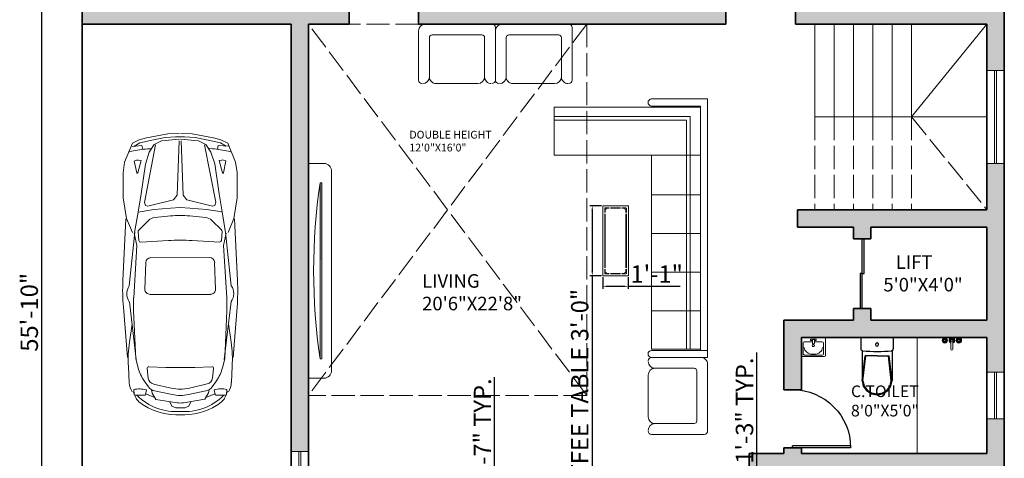
# Model space of a CAD drawing. Units: inches. Extents: x 4606 to 5879, y 1332 to 2209.
# Tile 3 of 7: x 4626 to 5136, y 1671 to 1897. Entities that reach past the tile are written whole.
import ezdxf

# ---------------------------------------------------------------- set-up
doc = ezdxf.new("R2010")
doc.units = ezdxf.units.IN
doc.linetypes.add('ACAD_ISO02W100', pattern=[15, 12, -3])
for name, color, linetype, lineweight in [('A-ANNO-DIMS', 2, 'Continuous', 18), ('A-AREA-IDEN', 7, 'Continuous', 18), ('A-DOOR', 4, 'Continuous', 25), ('A-EQPM', 9, 'Continuous', 18), ('A-FLOR-OVHD', 8, 'ACAD_ISO02W100', 13), ('A-FLOR-STRS', 7, 'Continuous', 20), ('A-FLOR-STRS-OVHD', 8, 'ACAD_ISO02W100', 13), ('A-FURN', 8, 'Continuous', 18), ('A-SITE-PARK', 8, 'Continuous', 13), ('A-WALL', 7, 'Continuous', 35), ('A-WALL-PATT', 252, 'Continuous', 13), ('window', 130, 'Continuous', 18), ('Сантехника', 9, 'Continuous', 18)]:
    doc.layers.add(name, color=color, linetype=linetype, lineweight=lineweight)
doc.layers.add('SANTEH', color=7, linetype='Continuous')
doc.styles.get("Standard").update_dxf_attribs({"font": 'arial.ttf'})
doc.dimstyles.new('ISO-25', dxfattribs={"dimtxt": 9, "dimasz": 2.5, "dimexe": 1.25, "dimexo": 0.625, "dimtad": 1, "dimlunit": 3, "dimtxsty": 'Standard', "dimcen": 2.5, "dimadec": 0, "dimazin": 0, "dimtfac": 1, "dimtmove": 0, "dimatfit": 3, "dimfxl": 1, "dimarcsym": 0})

# ---------------------------------------------------------------- blocks, each defined once
blk = doc.blocks.new('D2')
for p, q in [((0, 30), (0, 0)), ((1, 30), (1, 0)), ((0, 0), (1, 0))]:
    blk.add_line(p, q)
blk.add_arc((0, 0), 30, 0, 90)
blk = doc.blocks.new('WC 2 Symb_109')
at = {"layer": 'SANTEH'}
for p, q in [((0, 0), (0, 380)), ((0, 380), (132, 380)), ((154, 365), (507, 365)), ((506, 365), (216, 331)), ((506, 356), (216, 322)), ((216, 190), (216, 331)), ((216, 190), (216, 49)), ((154, 15), (507, 15)), ((506, 24), (216, 58)), ((506, 15), (216, 49)), ((0, 0), (132, 0))]:
    blk.add_line(p, q, dxfattribs=at)
for points in [[(155, 360), (154, 364), (152, 368), (150, 371), (147, 374), (144, 377), (140, 379), (137, 380), (132, 380)], [(155, 20), (159, 62), (161, 105), (163, 147), (164, 190), (163, 233), (161, 275), (159, 318), (155, 360)], [(506, 24), (565, 37), (616, 73), (649, 126), (661, 190), (649, 254), (616, 307), (565, 343), (506, 356)], [(507, 15), (569, 28), (622, 66), (658, 123), (670, 190), (658, 257), (622, 314), (569, 352), (507, 365)], [(132, 0), (136, 0), (140, 1), (144, 3), (147, 6), (150, 9), (152, 12), (154, 16), (155, 20)]]:
    blk.add_lwpolyline(points, dxfattribs=at)
blk.add_lwpolyline([(84, 208), (70, 203), (65, 190), (70, 177), (84, 172), (97, 177), (102, 190), (97, 203)], close=True, dxfattribs=at)
blk = doc.blocks.new('Faucet - Bathroom top')
for p, q in [((-4.107, 0.125), (-4.375, 0.125)), ((-3.75, 0.4788), (-3.75, 0.75)), ((-3.5, 0.482), (-3.5, 0.75)), ((-3.1461, 0.125), (-2.875, 0.125)), ((3.143, 0.125), (2.875, 0.125)), ((3.5, 0.4788), (3.5, 0.75)), ((3.75, 0.482), (3.75, 0.75)), ((4.1039, 0.125), (4.375, 0.125)), ((-4.1039, -0.125), (-4.375, -0.125)), ((-3.75, -0.4821), (-3.75, -0.75)), ((-3.5, -0.4789), (-3.5, -0.75)), ((-3.143, -0.125), (-2.875, -0.125)), ((-0.5, -0.8639), (-0.5, -4.5)), ((0.5, -4.5), (0.5, -0.8631)), ((3.1461, -0.125), (2.875, -0.125)), ((3.5, -0.4821), (3.5, -0.75)), ((3.75, -0.4789), (3.75, -0.75)), ((4.107, -0.125), (4.375, -0.125))]:
    blk.add_line(p, q)
for centre, radius in [((-3.625, 0), 1.375), ((-4.625, 0), 0.2795), ((-3.625, 0), 0.5), ((-3.625, 1), 0.2795), ((-2.625, 0), 0.2795), ((0, 0), 0.5), ((3.625, 0), 1.375), ((2.625, 0), 0.2795), ((3.625, 0), 0.5), ((3.625, 1), 0.2795), ((4.625, 0), 0.2795), ((-3.625, -1), 0.2795), ((3.625, -1), 0.2795)]:
    blk.add_circle(centre, radius)
for centre, radius, start, end in [((-3.625, 0), 1, 105.2407, 164.2093), ((-3.625, 0), 1, 16.44125, 74.07887), ((0, 0), 1.5, 289.6514, 250.3603), ((0, 0), 1, 300.3431, 239.7554), ((3.625, 0), 1, 106.12, 164.0884), ((3.625, 0), 1, 16.23422, 73.90469), ((-3.625, 0), 1, 196.2342, 253.9047), ((-3.625, 0), 1, 286.12, 344.0884), ((0, -4.5), 0.5, 180, 0), ((3.625, 0), 1, 196.4413, 254.0789), ((3.625, 0), 1, 285.2407, 344.2093)]:
    blk.add_arc(centre, radius, start, end)
blk = doc.blocks.new('Rac7')
at = {"color": 0}
for p, q in [((-39501, -24232), (-39501, -23830)), ((-39474, -23808), (-38988, -23808)), ((-39457, -23859), (-39457, -24115)), ((-39032, -23838), (-39430, -23838)), ((-39221, -23855), (-39241, -23855)), ((-39005, -24115), (-39005, -23859)), ((-39005, -23859), (-39005, -23859)), ((-38961, -23830), (-38961, -24232)), ((-38961, -24232), (-39501, -24232)), ((-39430, -24136), (-39253, -24136)), ((-39297, -24164), (-39253, -24164)), ((-39297, -24194), (-39297, -24164)), ((-39165, -24194), (-39297, -24194)), ((-39253, -24186), (-39253, -24094)), ((-39253, -24186), (-39209, -24186)), ((-39209, -24186), (-39209, -24094)), ((-39209, -24136), (-39032, -24136)), ((-39209, -24164), (-39165, -24164)), ((-39165, -24164), (-39165, -24194))]:
    blk.add_line(p, q, dxfattribs=at)
at = {"color": 0, "extrusion": (0, 0, -1)}
for centre, major_axis, start_param, end_param in [((-39474, -23830), (-27, 0), 0, 1.570796), ((-39430, -23859), (-27, 0), 0, 1.570796), ((-39241, -24007), (-194, 0), 0, 1.570796), ((-39221, -24007), (-194, 0), 1.570796, 3.141593), ((-39032, -23859), (-27, 0), 1.570796, 3.141593), ((-38988, -23830), (-27, 0), 1.570796, 3.141593), ((-39430, -24115), (-27, 0), -1.570796, 0), ((-39231, -24104), (-25.3, 0), 0.552816, 2.588777), ((-39032, -24115), (-27, 0), -3.141593, -1.570796)]:
    blk.add_ellipse(centre, major_axis=major_axis, ratio=0.785714, start_param=start_param, end_param=end_param, dxfattribs=at)
blk.add_ellipse((-39231, -24048), major_axis=(-27.9, 0), ratio=0.785714, dxfattribs=at)
blk = doc.blocks.new('TABLE-30A')
at = {"color": 0, "linetype": 'ByBlock'}
for p, q in [((0, 0), (0, 0.55)), ((0, 0.55), (1.5, 0.55)), ((0.051, 0.508), (0.042, 0.499)), ((0.042, 0.499), (0.042, 0.478)), ((0.042, 0.478), (0.072, 0.478)), ((0.042, 0.478), (0.042, 0.41)), ((0.072, 0.508), (0.051, 0.508)), ((0.051, 0.478), (0.051, 0.41)), ((0.072, 0.478), (0.072, 0.508)), ((0.072, 0.508), (0.14, 0.508)), ((0.072, 0.499), (0.14, 0.499)), ((1.331, 0.508), (0.169, 0.508)), ((1.331, 0.499), (0.169, 0.499)), ((1.428, 0.508), (1.36, 0.508)), ((1.428, 0.499), (1.36, 0.499)), ((1.428, 0.508), (1.428, 0.478)), ((1.449, 0.508), (1.428, 0.508)), ((1.428, 0.478), (1.458, 0.478)), ((1.458, 0.499), (1.449, 0.508)), ((1.449, 0.478), (1.449, 0.41)), ((1.458, 0.478), (1.458, 0.499)), ((1.458, 0.478), (1.458, 0.41)), ((1.5, 0.55), (1.5, 0)), ((0.042, 0.169), (0.042, 0.381)), ((0.051, 0.169), (0.051, 0.381)), ((1.449, 0.381), (1.449, 0.169)), ((1.458, 0.381), (1.458, 0.169)), ((1.5, 0), (0, 0)), ((0.042, 0.072), (0.042, 0.14)), ((0.042, 0.072), (0.042, 0.051)), ((0.072, 0.072), (0.042, 0.072)), ((0.042, 0.051), (0.051, 0.042)), ((0.051, 0.072), (0.051, 0.14)), ((0.051, 0.042), (0.072, 0.042)), ((0.072, 0.042), (0.072, 0.072)), ((0.072, 0.051), (0.14, 0.051)), ((0.072, 0.042), (0.14, 0.042)), ((0.169, 0.051), (1.331, 0.051)), ((0.169, 0.042), (1.331, 0.042)), ((1.428, 0.051), (1.36, 0.051)), ((1.428, 0.042), (1.36, 0.042)), ((1.428, 0.072), (1.428, 0.042)), ((1.458, 0.072), (1.428, 0.072)), ((1.428, 0.042), (1.449, 0.042)), ((1.449, 0.072), (1.449, 0.14)), ((1.449, 0.042), (1.458, 0.051)), ((1.458, 0.072), (1.458, 0.14)), ((1.458, 0.051), (1.458, 0.072))]:
    blk.add_line(p, q, dxfattribs=at)
blk = doc.blocks.new('sofa-27')
at = {"color": 0, "linetype": 'ByBlock'}
for p, q in [((0.0945, 0.5198), (0.459, 0.5198)), ((-0.0591, 0.0591), (-0.0591, 0.4902)), ((0.0354, 0.1181), (0.0354, 0.4607)), ((0.518, 0.1181), (0.518, 0.4607)), ((0.6125, 0.0295), (0.6125, 0.4902)), ((0.4944, 0.0945), (0.0591, 0.0945)), ((0.583, 0), (0, 0))]:
    blk.add_line(p, q, dxfattribs=at)
for centre, radius, start, end in [((-0.0295, 0.4902), 0.0295, 90, 180), ((-0.0236, 0.4607), 0.0591, 360, 90), ((0.0945, 0.4607), 0.0591, 90, 180), ((0.459, 0.4607), 0.0591, 0, 90), ((0.5771, 0.4607), 0.0591, 90, 180), ((0.583, 0.4902), 0.0295, 0, 90), ((0.0591, 0.1181), 0.0236, 180, 270), ((0.4944, 0.1181), 0.0236, 270, 0), ((0, 0.0591), 0.0591, 180, 270), ((0.583, 0.0295), 0.0295, 270, 0)]:
    blk.add_arc(centre, radius, start, end, dxfattribs=at)
blk = doc.blocks.new('A$C4A3239E3')
for p, q in [((1.251, 1.634), (2.152, 1.68)), ((2.545, 1.674), (3.282, 1.615)), ((3.41, 1.602), (3.649, 1.59)), ((0.136, 1.429), (0.187, 1.515)), ((0.175, 1.399), (0.187, 1.541)), ((0.266, 1.579), (0.259, 1.549)), ((0.396, 1.412), (0.388, 1.449)), ((0.39, 1.477), (0.402, 1.511)), ((0.576, 1.46), (0.396, 1.412)), ((0.402, 1.511), (0.575, 1.474)), ((1.45, 1.506), (1.149, 1.455)), ((1.272, 1.303), (1.413, 1.446)), ((1.433, 1.454), (1.567, 1.444)), ((1.443, 1.502), (2.231, 1.588)), ((1.461, 1.515), (1.641, 1.474)), ((1.641, 1.474), (2.408, 1.522)), ((2.463, 1.587), (3.312, 1.486)), ((2.597, 1.524), (3.301, 1.494)), ((2.788, 1.546), (3.057, 1.586)), ((3.301, 1.494), (3.432, 1.46)), ((3.822, 1.52), (3.752, 1.525)), ((3.781, 1.532), (3.813, 1.518)), ((3.833, 1.363), (3.833, 1.508)), ((3.838, 1.508), (3.867, 1.496)), ((0.09, 1.227), (0.136, 1.429)), ((0.231, 1.387), (0.175, 1.399)), ((0.224, 1.314), (0.221, 1.265)), ((1.59, 1.418), (1.567, 1.013)), ((1.89, 1.345), (2.279, 1.358)), ((3.416, 1.302), (3.429, 1.052)), ((3.443, 1.328), (3.584, 1.312)), ((3.622, 1.372), (3.711, 1.31)), ((3.756, 1.339), (3.823, 1.351)), ((3.814, 1.35), (3.869, 1.214)), ((0.056, 1.059), (0.09, 1.227)), ((1.207, 0.98), (1.229, 1.212)), ((1.819, 0.408), (1.818, 1.271)), ((2.356, 1.283), (2.357, 0.397)), ((3.669, 1.236), (3.73, 0.976)), ((3.753, 1.264), (3.801, 1.255)), ((3.771, 1.218), (3.825, 0.963)), ((3.801, 1.255), (3.894, 1.199)), ((3.894, 1.199), (3.945, 0.89)), ((0.048, 0.904), (0.056, 1.059)), ((3.429, 1.052), (3.429, 0.843)), ((3.929, 0.994), (3.993, 0.967)), ((3.993, 0.967), (4.017, 0.906)), ((4.017, 0.906), (4.021, 0.842)), ((0.048, 0.772), (0.057, 0.617)), ((3.43, 0.631), (3.429, 0.84)), ((3.895, 0.484), (3.945, 0.793)), ((3.994, 0.717), (4.017, 0.778)), ((4.017, 0.778), (4.021, 0.842)), ((0.057, 0.617), (0.091, 0.45)), ((1.208, 0.698), (1.23, 0.466)), ((1.591, 0.261), (1.567, 0.666)), ((3.417, 0.38), (3.43, 0.631)), ((3.67, 0.447), (3.73, 0.707)), ((3.772, 0.465), (3.825, 0.721)), ((3.929, 0.689), (3.994, 0.717)), ((0.091, 0.45), (0.137, 0.247)), ((3.802, 0.428), (3.895, 0.484)), ((3.815, 0.333), (3.869, 0.469)), ((0.232, 0.29), (0.176, 0.277)), ((0.225, 0.362), (0.222, 0.411)), ((1.273, 0.375), (1.415, 0.232)), ((1.891, 0.334), (2.28, 0.323)), ((3.444, 0.354), (3.585, 0.371)), ((3.623, 0.311), (3.712, 0.373)), ((3.754, 0.419), (3.802, 0.428)), ((3.757, 0.344), (3.824, 0.333)), ((3.834, 0.32), (3.835, 0.175)), ((0.137, 0.247), (0.188, 0.161)), ((0.176, 0.277), (0.188, 0.136)), ((0.397, 0.265), (0.389, 0.228)), ((0.391, 0.2), (0.403, 0.166)), ((0.577, 0.217), (0.397, 0.265)), ((0.403, 0.166), (0.577, 0.203)), ((1.451, 0.172), (1.15, 0.223)), ((1.434, 0.225), (1.568, 0.235)), ((1.444, 0.176), (2.233, 0.092)), ((1.462, 0.164), (1.642, 0.205)), ((1.642, 0.205), (2.409, 0.158)), ((2.464, 0.094), (3.313, 0.196)), ((2.598, 0.156), (3.302, 0.188)), ((3.302, 0.188), (3.433, 0.223)), ((3.823, 0.163), (3.753, 0.158)), ((3.783, 0.151), (3.814, 0.165)), ((3.839, 0.175), (3.868, 0.188)), ((0.268, 0.097), (0.261, 0.127)), ((1.252, 0.045), (2.154, 0)), ((2.546, 0.006), (3.283, 0.067)), ((2.789, 0.135), (3.058, 0.096)), ((3.412, 0.08), (3.651, 0.093))]:
    blk.add_line(p, q)
for points in [[(0, 0.848), (0.005, 1.016), (0.062, 1.33), (0.09, 1.438), (0.141, 1.536), (0.419, 1.653), (0.572, 1.674), (0.94, 1.674), (1.246, 1.627), (1.45, 1.541)], [(0.081, 0.844), (0.109, 1.11), (0.161, 1.218), (0.274, 1.291), (0.446, 1.347), (0.881, 1.409), (1.149, 1.455), (1.112, 1.224), (1.093, 0.981), (1.085, 0.839)], [(0.164, 1.198), (1.007, 1.364), (1.054, 1.346), (1.062, 1.312), (0.971, 0.937), (0.904, 0.882), (0.106, 0.853)], [(0, 0.828), (0.006, 0.66), (0.063, 0.346), (0.092, 0.239), (0.143, 0.14), (0.42, 0.024), (0.574, 0.003), (0.942, 0.003), (1.247, 0.051), (1.451, 0.138)], [(0.081, 0.832), (0.109, 0.566), (0.162, 0.458), (0.275, 0.386), (0.447, 0.33), (0.882, 0.268), (1.15, 0.223), (1.113, 0.454), (1.094, 0.696), (1.085, 0.839)], [(0.165, 0.478), (1.008, 0.314), (1.055, 0.332), (1.063, 0.366), (0.971, 0.741), (0.904, 0.796), (0.106, 0.823)]]:
    blk.add_lwpolyline(points)
for centre, radius, start, end in [((2.305, -1.296), 2.98, 85.3952, 92.9452), ((2.346, 1.423), 0.202, 54.6492, 124.7769), ((3.317, -0.183), 1.788, 86.9998, 98.3676), ((3.635, 1.312), 0.278, 57.3299, 87.1824), ((1.71, 1.212), 1.49, 166.9166, 176.0811), ((0.436, 1.46), 0.0497, 159.9787, 192.5384), ((0.574, 1.467), 0.00745, 284.96, 78.1125), ((1.431, 1.429), 0.0248, 85.7151, 135.3046), ((2.521, -0.262), 1.788, 87.5491, 93.6237), ((3.28, 0.883), 0.596, 55.07, 75.2551), ((4.097, 1.439), 0.356, 166.0961, 196.3535), ((3.821, 1.508), 0.0124, 0, 86.3304), ((3.247, 0.896), 0.828, 356.2451, 44.5195), ((3.809, 1.358), 0.149, 46.3836, 67.2014), ((3.618, 1.158), 0.426, 30.4577, 46.3836), ((1.378, 1.198), 0.149, 135.3046, 174.6214), ((1.565, 1.419), 0.0248, 356.7256, 85.7151), ((1.892, 1.271), 0.0745, 91.8201, 179.9989), ((2.281, 1.283), 0.0745, 359.9245, 91.8201), ((3.441, 1.304), 0.0248, 83.376, 183.115), ((3.573, 1.213), 0.0993, 13.1226, 83.376), ((3.625, 1.188), 0.149, 11.7694, 55.07), ((3.821, 1.363), 0.0124, 279.6077, 0), ((3.132, 0.872), 0.989, 358.0694, 30.4577), ((4.542, 0.842), 2.98, 176.7256, 183.3874), ((1.238, 0.839), 1.192, 176.8942, 183.2188), ((2.691, 0.84), 1.49, 174.6214, 185.4916), ((3.149, 0.841), 0.596, 346.9903, 13.1226), ((3.241, 0.841), 0.596, 348.3436, 11.7694), ((3.651, 0.841), 0.298, 350.7246, 9.3883), ((3.247, 0.786), 0.828, 315.5935, 3.8679), ((3.133, 0.809), 0.989, 329.6553, 2.0435), ((1.378, 0.48), 0.149, 185.4916, 224.8083), ((3.573, 0.469), 0.0993, 276.737, 346.9903), ((3.626, 0.495), 0.149, 305.0429, 348.3436), ((1.711, 0.467), 1.49, 184.0319, 193.1964), ((1.893, 0.409), 0.0745, 180.1141, 268.2929), ((2.282, 0.397), 0.0745, 268.2929, 0.1885), ((3.441, 0.379), 0.0248, 176.9979, 276.737), ((3.281, 0.799), 0.596, 284.8579, 305.0429), ((4.098, 0.244), 0.356, 163.7595, 194.0169), ((3.822, 0.32), 0.0124, 0.113, 80.5053), ((3.619, 0.525), 0.426, 313.7293, 329.6553), ((0.438, 0.217), 0.0497, 167.5746, 200.1342), ((0.575, 0.21), 0.00745, 282.0005, 75.153), ((1.432, 0.249), 0.0248, 224.8083, 274.3979), ((1.566, 0.26), 0.0248, 274.3979, 3.3874), ((2.518, 1.942), 1.788, 266.4893, 272.5638), ((3.822, 0.175), 0.0124, 273.7825, 0.113), ((3.81, 0.325), 0.149, 292.9116, 313.7293), ((2.301, 2.976), 2.98, 267.1678, 274.7177), ((2.347, 0.258), 0.202, 235.336, 305.4638), ((3.315, 1.865), 1.788, 261.7454, 273.1132), ((3.636, 0.371), 0.278, 272.9306, 302.783)]:
    blk.add_arc(centre, radius, start, end)
blk = doc.blocks.new('*D24')
at = {"layer": 'A-ANNO-DIMS', "color": 0, "lineweight": -2, "transparency": 16777216}
for p, q in [((4658.23, 2081.24), (4636.6, 2081.24)), ((4637.85, 2078.74), (4637.85, 1413.74)), ((4658.23, 1411.24), (4636.6, 1411.24))]:
    blk.add_line(p, q, dxfattribs=at)
at = {"layer": 'A-ANNO-DIMS', "color": 0, "transparency": 16777216}
for points in [[(4637.43, 2078.74), (4638.26, 2078.74), (4637.85, 2081.24)], [(4637.43, 1413.74), (4638.26, 1413.74), (4637.85, 1411.24)]]:
    blk.add_solid(points, dxfattribs=at)
at = {"layer": 'Defpoints', "color": 0, "transparency": 16777216}
for p in [(4658.85, 2081.24), (4637.85, 1411.24), (4658.85, 1411.24)]:
    blk.add_point(p, dxfattribs=at)
at = {"layer": 'A-ANNO-DIMS', "color": 0, "transparency": 16777216, "insert": (4632.62, 1746.24), "char_height": 9, "attachment_point": 5, "rotation": 90}
blk.add_mtext('55\'-10"', dxfattribs=at)
blk = doc.blocks.new('GLAZING-72IN')
for p, q in [((0, 0), (0, 72)), ((1, 0), (1, 72))]:
    blk.add_line(p, q)
blk = doc.blocks.new('GLAZING-24IN')
for p, q in [((0, 0), (0, 24)), ((1, 0), (1, 24))]:
    blk.add_line(p, q)
blk = doc.blocks.new('GLAZING-48IN')
for p, q in [((0, 0), (0, 48)), ((1, 0), (1, 48))]:
    blk.add_line(p, q)
blk = doc.blocks.new('LIFT-DOOR-36IN')
for p, q in [((1, 0), (1, 36)), ((2, 18), (2, 36)), ((1, 18), (0, 18)), ((0, 18), (0, 0)), ((1, 18), (2, 18))]:
    blk.add_line(p, q)
blk = doc.blocks.new('*D83')
at = {"layer": 'A-ANNO-DIMS', "color": 0, "lineweight": -2, "transparency": 16777216}
for p, q in [((5007.89, 1624.4), (5007.89, 1725.52)), ((5009.49, 1624.4), (5006.64, 1624.4)), ((5007.89, 1612.06), (5007.89, 1621.9)), ((5009.49, 1609.56), (5006.64, 1609.56))]:
    blk.add_line(p, q, dxfattribs=at)
at = {"layer": 'A-ANNO-DIMS', "color": 0, "transparency": 16777216}
for points in [[(5007.47, 1621.9), (5008.31, 1621.9), (5007.89, 1624.4)], [(5007.47, 1612.06), (5008.31, 1612.06), (5007.89, 1609.56)]]:
    blk.add_solid(points, dxfattribs=at)
at = {"layer": 'Defpoints', "color": 0, "transparency": 16777216}
for p in [(5007.89, 1624.4), (5010.11, 1624.4), (5010.11, 1609.56)]:
    blk.add_point(p, dxfattribs=at)
at = {"layer": 'A-ANNO-DIMS', "color": 0, "transparency": 16777216, "insert": (5002.61, 1676.21), "char_height": 9, "attachment_point": 5, "rotation": 90}
blk.add_mtext('CHAIR 1\'-3" TYP.', dxfattribs=at)
blk = doc.blocks.new('*D88')
at = {"layer": 'A-ANNO-DIMS', "color": 0, "lineweight": -2, "transparency": 16777216}
for p, q in [((4872.19, 1654), (4872.19, 1712.76)), ((4866.85, 1654), (4873.44, 1654)), ((4872.19, 1625.74), (4872.19, 1651.5)), ((4866.85, 1623.24), (4873.44, 1623.24))]:
    blk.add_line(p, q, dxfattribs=at)
at = {"layer": 'A-ANNO-DIMS', "color": 0, "transparency": 16777216}
for points in [[(4871.77, 1651.5), (4872.6, 1651.5), (4872.19, 1654)], [(4871.77, 1625.74), (4872.6, 1625.74), (4872.19, 1623.24)]]:
    blk.add_solid(points, dxfattribs=at)
at = {"layer": 'Defpoints', "color": 0, "transparency": 16777216}
for p in [(4866.23, 1654), (4872.19, 1654), (4866.23, 1623.24)]:
    blk.add_point(p, dxfattribs=at)
at = {"layer": 'A-ANNO-DIMS', "color": 0, "transparency": 16777216, "insert": (4867.04, 1684.63), "char_height": 9, "attachment_point": 5, "rotation": 90}
blk.add_mtext('2\'-7" TYP.', dxfattribs=at)
blk = doc.blocks.new('*D105')
at = {"layer": 'A-ANNO-DIMS', "color": 0, "lineweight": -2, "transparency": 16777216}
for p, q in [((4927.48, 1801.23), (4921.43, 1801.23)), ((4922.68, 1798.73), (4922.68, 1767.59)), ((4927.48, 1765.09), (4921.43, 1765.09)), ((4922.68, 1765.09), (4922.68, 1639.71))]:
    blk.add_line(p, q, dxfattribs=at)
at = {"layer": 'A-ANNO-DIMS', "color": 0, "transparency": 16777216}
for points in [[(4922.27, 1798.73), (4923.1, 1798.73), (4922.68, 1801.23)], [(4922.27, 1767.59), (4923.1, 1767.59), (4922.68, 1765.09)]]:
    blk.add_solid(points, dxfattribs=at)
at = {"layer": 'Defpoints', "color": 0, "transparency": 16777216}
for p in [(4928.1, 1801.23), (4922.68, 1765.09), (4928.1, 1765.09)]:
    blk.add_point(p, dxfattribs=at)
at = {"layer": 'A-ANNO-DIMS', "color": 0, "transparency": 16777216, "insert": (4917.4, 1701.15), "char_height": 9, "attachment_point": 5, "rotation": 90}
blk.add_mtext('COFFEE TABLE 3\'-0"', dxfattribs=at)
blk = doc.blocks.new('*D106')
at = {"layer": 'A-ANNO-DIMS', "color": 0, "lineweight": -2, "transparency": 16777216}
for p, q in [((4928.1, 1764.47), (4928.1, 1758.42)), ((4941.35, 1764.47), (4941.35, 1758.42)), ((4930.6, 1759.67), (4938.85, 1759.67)), ((4941.35, 1759.67), (4968.18, 1759.67))]:
    blk.add_line(p, q, dxfattribs=at)
at = {"layer": 'A-ANNO-DIMS', "color": 0, "transparency": 16777216}
for points in [[(4930.6, 1760.09), (4930.6, 1759.26), (4928.1, 1759.67)], [(4938.85, 1760.09), (4938.85, 1759.26), (4941.35, 1759.67)]]:
    blk.add_solid(points, dxfattribs=at)
at = {"layer": 'Defpoints', "color": 0, "transparency": 16777216}
for p in [(4928.1, 1765.09), (4941.35, 1765.09), (4941.35, 1759.67)]:
    blk.add_point(p, dxfattribs=at)
at = {"layer": 'A-ANNO-DIMS', "color": 0, "transparency": 16777216, "insert": (4956.02, 1764.82), "char_height": 9, "attachment_point": 5}
blk.add_mtext('1\'-1"', dxfattribs=at)

msp = doc.modelspace()

# ---------------------------------------------------------------- hatches: boundary and pattern name
at = {"layer": 'A-EQPM', "transparency": 33554687}
h = msp.add_hatch(color=256, dxfattribs=at)
h.dxf.hatch_style = 1
h.paths.add_polyline_path([(4782.85, 1813.179), (4781.85, 1813.179), (4781.85, 1773.179), (4782.85, 1773.179)])
at = {"layer": 'A-WALL-PATT', "transparency": 33554687}
h = msp.add_hatch(color=256, dxfattribs=at)
h.dxf.hatch_style = 1
h.paths.add_polyline_path([(4715.85, 2081.239), (4658.85, 2081.239), (4658.85, 2054.239), (4667.85, 2054.239), (4667.85, 2072.239), (4715.85, 2072.239)])
h.paths.add_polyline_path([(4868.85, 2081.239), (4787.85, 2081.239), (4787.85, 2072.239), (4835.85, 2072.239), (4835.85, 1955.239), (4844.85, 1955.239), (4844.85, 1970.239), (4850.85, 1970.239), (4850.85, 1976.239), (4844.85, 1976.239), (4844.85, 2072.239), (4868.85, 2072.239)])
h.paths.add_polyline_path([(4940.85, 2081.239), (4892.85, 2081.239), (4892.85, 2072.239), (4916.85, 2072.239), (4916.85, 1976.239), (4880.85, 1976.239), (4880.85, 1970.239), (4916.85, 1970.239), (4916.85, 1904.239), (4844.85, 1904.239), (4844.85, 1925.239), (4835.85, 1925.239), (4835.85, 1904.239), (4832.85, 1904.239), (4832.85, 1895.239), (4919.85, 1895.239), (4991.85, 1895.239), (4991.85, 1904.239), (4988.85, 1904.239), (4988.85, 1925.239), (4982.85, 1925.239), (4982.85, 1904.239), (4922.85, 1904.239), (4922.85, 1970.239), (4946.85, 1970.239), (4946.85, 1976.239), (4922.85, 1976.239), (4922.85, 2072.239), (4940.85, 2072.239)])
h.paths.add_polyline_path([(5021.85, 2081.239), (4964.85, 2081.239), (4964.85, 2072.239), (4982.85, 2072.239), (4982.85, 1976.239), (4976.85, 1976.239), (4976.85, 1970.239), (4982.85, 1970.239), (4982.85, 1955.239), (4988.85, 1955.239), (4988.85, 2072.239), (5021.85, 2072.239)])
h.paths.add_polyline_path([(5135.85, 2081.239), (5093.85, 2081.239), (5093.85, 2072.239), (5126.85, 2072.239), (5126.85, 2054.239), (5135.85, 2054.239)])
h.paths.add_polyline_path([(5135.85, 2006.239), (5126.85, 2006.239), (5126.85, 1976.239), (5135.85, 1976.239)])
h.paths.add_polyline_path([(5135.85, 1928.239), (5126.85, 1928.239), (5126.85, 1904.239), (5027.85, 1904.239), (5027.85, 1895.239), (5126.85, 1895.239), (5126.85, 1871.239), (5135.85, 1871.239)])
h.paths.add_polyline_path([(4796.85, 1904.239), (4667.85, 1904.239), (4667.85, 1922.239), (4658.85, 1922.239), (4658.85, 1895.239), (4766.85, 1895.239), (4766.85, 1674.239), (4775.85, 1674.239), (4775.85, 1895.239), (4796.85, 1895.239)])
h.paths.add_polyline_path([(4667.85, 2006.239), (4658.85, 2006.239), (4658.85, 1970.239), (4667.85, 1970.239)])
h.paths.add_polyline_path([(4880.85, 1545.239), (4940.85, 1545.239), (4940.85, 1542.239), (4949.85, 1542.239), (4949.85, 1566.239), (4940.85, 1566.239), (4940.85, 1554.239), (4880.85, 1554.239), (4880.85, 1614.239), (4940.85, 1614.239), (4940.85, 1602.239), (4949.85, 1602.239), (4949.85, 1623.239), (4866.739, 1623.239), (4826.85, 1623.239), (4826.85, 1614.239), (4871.85, 1614.239), (4871.85, 1554.239), (4826.85, 1554.239), (4826.85, 1545.239), (4871.85, 1545.239), (4871.85, 1411.239), (4997.85, 1411.239), (4997.85, 1420.239), (4949.85, 1420.239), (4949.85, 1512.239), (4940.85, 1512.239), (4940.85, 1420.239), (4880.85, 1420.239)])
h.paths.add_polyline_path([(5102.85, 1446.239), (5093.85, 1446.239), (5093.85, 1420.239), (5045.85, 1420.239), (5045.85, 1411.239), (5102.85, 1411.239)])
h.paths.add_polyline_path([(5102.85, 1591.739), (5093.85, 1591.739), (5093.85, 1542.239), (5102.85, 1542.239)])
h.paths.add_polyline_path([(5135.85, 1691.239), (5126.85, 1691.239), (5126.85, 1673.239), (5030.85, 1673.239), (5030.85, 1676.239), (5021.85, 1676.239), (5021.85, 1673.239), (5003.85, 1673.239), (5003.85, 1664.239), (5093.85, 1664.239), (5093.85, 1639.739), (5102.85, 1639.739), (5102.85, 1664.239), (5135.85, 1664.239)])
h.paths.add_polyline_path([(5135.85, 1823.239), (5126.85, 1823.239), (5126.85, 1799.239), (5028.85, 1799.239), (5028.85, 1790.239), (5057.85, 1790.239), (5057.85, 1784.239), (5066.85, 1784.239), (5066.85, 1790.239), (5126.85, 1790.239), (5126.85, 1742.239), (5066.85, 1742.239), (5066.85, 1748.239), (5057.85, 1748.239), (5057.85, 1742.239), (5021.85, 1742.239), (5021.85, 1706.239), (5030.85, 1706.239), (5030.85, 1733.239), (5126.85, 1733.239), (5126.85, 1715.239), (5135.85, 1715.239)])
h.paths.add_polyline_path([(4775.85, 1602.239), (4766.85, 1602.239), (4766.85, 1474.239), (4775.85, 1474.239), (4775.85, 1545.239), (4778.85, 1545.239), (4778.85, 1554.239), (4775.85, 1554.239)])
h.paths.add_polyline_path([(4692.58, 1635.003), (4749.356, 1635.003), (4749.356, 1665.418), (4692.58, 1665.418)], flags=9)

# ---------------------------------------------------------------- linework, layer by layer
at = {"layer": 'A-EQPM'}
for p, q in [((4775.85, 1823.179), (4783.85, 1823.179)), ((4787.85, 1819.179), (4787.85, 1716.179)), ((4781.85, 1813.179), (4782.85, 1813.179)), ((4781.85, 1722.179), (4781.85, 1813.179)), ((4782.85, 1722.179), (4782.85, 1813.179)), ((4781.85, 1722.179), (4782.85, 1722.179)), ((4775.85, 1712.179), (4783.85, 1712.179))]:
    msp.add_line(p, q, dxfattribs=at)
for centre, radius, start, end in [((4783.85, 1819.179), 4, 0, 90), ((5095.336, 1767.679), 316.77, 171.74163, 188.25837), ((4783.85, 1716.179), 4, 270, 0)]:
    msp.add_arc(centre, radius, start, end, dxfattribs=at)
at = {"layer": 'A-FLOR-OVHD'}
for p, q in [((4919.85, 1703.239), (4775.85, 1895.239)), ((4919.85, 1895.239), (4775.85, 1703.239))]:
    msp.add_line(p, q, dxfattribs=at)
msp.add_lwpolyline([(4775.85, 1895.239), (4919.85, 1895.239), (4919.85, 1703.239), (4775.85, 1703.239)], close=True, dxfattribs=at)
at = {"layer": 'A-FLOR-STRS'}
for p, q in [((5037.85, 1847.239), (5037.85, 1895.239)), ((5047.85, 1847.239), (5047.85, 1895.239)), ((5057.85, 1847.239), (5057.85, 1895.239)), ((5067.85, 1847.239), (5067.85, 1895.239)), ((5077.85, 1847.239), (5077.85, 1895.239)), ((5087.85, 1847.239), (5087.85, 1895.239)), ((5087.85, 1847.239), (5126.85, 1895.239)), ((5037.85, 1847.239), (5126.85, 1847.239))]:
    msp.add_line(p, q, dxfattribs=at)
at = {"layer": 'A-FLOR-STRS-OVHD'}
for p, q in [((5037.85, 1847.239), (5037.85, 1799.239)), ((5047.85, 1847.239), (5047.85, 1799.239)), ((5057.85, 1847.239), (5057.85, 1799.239)), ((5067.85, 1847.239), (5067.85, 1799.239)), ((5077.85, 1847.239), (5077.85, 1799.239)), ((5087.85, 1847.239), (5087.85, 1799.239)), ((5087.85, 1847.239), (5126.85, 1799.239))]:
    msp.add_line(p, q, dxfattribs=at)
at = {"layer": 'A-FURN'}
for p, q in [((4953.363, 1856.501), (4982.384, 1856.501)), ((4982.384, 1856.501), (4982.384, 1722.883)), ((4902.901, 1852.267), (4902.901, 1827.48)), ((4978.757, 1852.267), (4902.901, 1852.267)), ((4953.363, 1852.874), (4978.757, 1852.874)), ((4978.757, 1852.874), (4978.757, 1726.511)), ((4902.901, 1847.432), (4973.315, 1847.432)), ((4902.901, 1845.618), (4971.501, 1845.618)), ((4971.501, 1845.618), (4971.501, 1727.117)), ((4973.315, 1847.432), (4973.315, 1727.117)), ((4978.757, 1827.48), (4902.901, 1827.48)), ((4953.363, 1727.117), (4953.363, 1827.48)), ((4978.757, 1806.923), (4953.363, 1806.923)), ((4978.757, 1786.971), (4953.363, 1786.971)), ((4978.757, 1767.02), (4953.363, 1767.02)), ((4978.757, 1747.068), (4953.363, 1747.068)), ((4978.757, 1727.117), (4953.363, 1727.117)), ((4978.757, 1727.117), (4953.363, 1727.117)), ((4982.384, 1726.511), (4953.363, 1726.511)), ((4982.384, 1722.883), (4953.363, 1722.883))]:
    msp.add_line(p, q, dxfattribs=at)
for centre in [(4953.363, 1854.687), (4953.363, 1724.697)]:
    msp.add_arc(centre, 1.814, 90, 270, dxfattribs=at)
at = {"layer": 'A-WALL'}
for p, q in [((4796.85, 1904.239), (4796.85, 1895.239)), ((4832.85, 1904.239), (4832.85, 1895.239)), ((4991.85, 1904.239), (4991.85, 1895.239)), ((5027.85, 1904.239), (5027.85, 1895.239)), ((4766.85, 1895.239), (4658.85, 1895.239)), ((4766.85, 1895.239), (4766.85, 1474.239)), ((4775.85, 1895.239), (4775.85, 1554.239)), ((4796.85, 1895.239), (4775.85, 1895.239)), ((4991.85, 1895.239), (4832.85, 1895.239)), ((5126.85, 1895.239), (5027.85, 1895.239)), ((5126.85, 1799.239), (5126.85, 1895.239)), ((5126.85, 1799.239), (5028.85, 1799.239)), ((5028.85, 1799.239), (5028.85, 1790.239)), ((5057.85, 1790.239), (5028.85, 1790.239)), ((5057.85, 1784.239), (5057.85, 1790.239)), ((5126.85, 1790.239), (5066.85, 1790.239)), ((5066.85, 1784.239), (5066.85, 1790.239)), ((5126.85, 1742.239), (5126.85, 1790.239)), ((5066.85, 1784.239), (5057.85, 1784.239)), ((5057.85, 1742.239), (5057.85, 1748.239)), ((5066.85, 1748.239), (5057.85, 1748.239)), ((5066.85, 1742.239), (5066.85, 1748.239)), ((5057.85, 1742.239), (5021.85, 1742.239)), ((5021.85, 1706.239), (5021.85, 1742.239)), ((5126.85, 1742.239), (5066.85, 1742.239)), ((5126.85, 1733.239), (5030.85, 1733.239)), ((5030.85, 1706.239), (5030.85, 1733.239)), ((5126.85, 1673.239), (5126.85, 1733.239)), ((5030.85, 1706.239), (5021.85, 1706.239)), ((5021.85, 1673.239), (5021.85, 1676.239)), ((5030.85, 1676.239), (5021.85, 1676.239)), ((5030.85, 1673.239), (5030.85, 1676.239)), ((5003.85, 1664.239), (5003.85, 1673.239)), ((5021.85, 1673.239), (5003.85, 1673.239)), ((5126.85, 1673.239), (5030.85, 1673.239))]:
    msp.add_line(p, q, dxfattribs=at)
msp.add_lwpolyline([(5135.85, 1664.239), (5135.85, 2081.239), (4658.85, 2081.239), (4658.85, 1411.239), (5102.85, 1411.239)], dxfattribs=at)
at = {"layer": 'window'}
for p, q in [((5126.85, 1871.239), (5135.85, 1871.239)), ((5126.85, 1823.239), (5135.85, 1823.239)), ((5126.85, 1715.239), (5135.85, 1715.239)), ((5126.85, 1691.239), (5135.85, 1691.239)), ((4766.85, 1674.239), (4775.85, 1674.239))]:
    msp.add_line(p, q, dxfattribs=at)
at = {"layer": 'Сантехника'}
msp.add_line((5090.85, 1673.239), (5090.85, 1733.239), dxfattribs=at)

# ---------------------------------------------------------------- block references
at = {"layer": 'A-DOOR'}
msp.add_blockref('LIFT-DOOR-36IN', (5061.35, 1748.239), dxfattribs=at)
at = {"layer": 'A-DOOR', "xscale": -1, "rotation": 270}
msp.add_blockref('D2', (5026.35, 1676.239), dxfattribs=at)
at = {"layer": 'A-FURN'}
for name, p, xscale, yscale, zscale, rotation in [('sofa-27', (4836.327, 1895.239), -59.17827105340016, 59.17827105340016, 59.17827105340016, 180.0000000000332), ('sofa-27', (4876.069, 1895.239), -59.17827105340016, 59.17827105340016, 59.17827105340016, 180.0000000000332), ('TABLE-30A', (4928.104, 1801.225), 24.08863485716172, 24.08863485716172, 24.08863485716172, 270), ('sofa-27', (4982.373, 1719.388), -59.17827105340016, 59.17827105340016, 59.17827105340016, 90.00000000003318)]:
    msp.add_blockref(name, p, dxfattribs=dict(at, xscale=xscale, yscale=yscale, zscale=zscale, rotation=rotation))
at = {"layer": 'A-SITE-PARK', "xscale": 35.27598425228, "yscale": 35.27598425228, "zscale": 35.27598425228, "rotation": 270}
msp.add_blockref('A$C4A3239E3', (4679.899, 1838.634), dxfattribs=at)
at = {"layer": 'window'}
for name, p in [('GLAZING-48IN', (5130.85, 1823.239)), ('GLAZING-24IN', (5130.85, 1691.239)), ('GLAZING-72IN', (4770.85, 1602.239))]:
    msp.add_blockref(name, p, dxfattribs=at)
at = {"layer": 'Сантехника'}
for name, p, xscale, yscale, zscale, rotation in [('Rac7', (4130.473, 1173.247), 0.0231094998546128, 0.0231094998546128, 0.0231094998546128, 179.9999999999958), ('WC 2 Symb_109', (5061.644, 1733.239), 0.0441898926459964, 0.0441898926459964, 0.0441898926459964, 269.9999999999999)]:
    msp.add_blockref(name, p, dxfattribs=dict(at, xscale=xscale, yscale=yscale, zscale=zscale, rotation=rotation))
msp.add_blockref('Faucet - Bathroom top', (5108.73, 1731.739), dxfattribs=at)

# ---------------------------------------------------------------- texts
at = {"layer": 'A-AREA-IDEN', "attachment_point": 1}
for s, insert, char_height in [('{\\fTimes New Roman|b0|i0|c0|p18;DOUBLE HEIGHT\\P12\'0"X16\'0"}', (4828.097, 1840.052), 4), ('{\\fTimes New Roman|b0|i0|c0|p18;   LIFT\\P5\'0"X4\'0"}', (5073.274, 1775.694), 7), ('{\\fTimes New Roman|b0|i0|c0|p18;LIVING\\P20\'6"X22\'8"}', (4834.683, 1765.94), 7), ('{\\fTimes New Roman|b0|i0|c0|p18;C.TOILET\\P8\'0"X5\'0"}', (5056.532, 1708.408), 6)]:
    msp.add_mtext_dynamic_manual_height_columns(s, width=80.30411, gutter_width=12.5, heights=[0], dxfattribs=dict(at, insert=insert, char_height=char_height))

# ---------------------------------------------------------------- dimensions: what is measured, and where the dimension line sits
at = {"layer": 'A-ANNO-DIMS'}
dim = msp.add_linear_dim(base=(4637.845, 1411.239), p1=(4658.85, 2081.239), p2=(4658.85, 1411.239), angle=90, dimstyle='ISO-25', override={"dimclrd": 0, "dimclre": 0, "dimclrt": 0}, dxfattribs=at)
dim.commit()
dim.dimension.update_dxf_attribs({"geometry": '*D24', "text_midpoint": (4632.625, 1746.239)})
for base, p1, p2, angle, text, picture, middle in [((4922.684, 1765.092), (4928.104, 1801.225), (4928.104, 1765.092), 270, 'COFFEE TABLE <>', '*D105', (4917.399, 1701.153)), ((5007.889, 1624.402), (5010.115, 1609.564), (5010.115, 1624.402), 90, 'CHAIR <> TYP.', '*D83', (5002.608, 1676.21)), ((4872.186, 1653.997), (4866.225, 1623.239), (4866.225, 1653.997), 90, '<> TYP.', '*D88', (4867.04, 1684.628))]:
    dim = msp.add_linear_dim(base=base, p1=p1, p2=p2, angle=angle, text=text, dimstyle='ISO-25', override={"dimdec": 1, "dimlfac": 1, "dimrnd": 0, "dimzin": 1, "dimdsep": 46, "dimlunit": 4, "dimfrac": 2}, dxfattribs=at)
    dim.commit()
    dim.dimension.update_dxf_attribs({"geometry": picture, "text_midpoint": middle})
dim = msp.add_linear_dim(base=(4941.353, 1759.672), p1=(4928.104, 1765.092), p2=(4941.353, 1765.092), dimstyle='ISO-25', override={"dimdec": 1, "dimlfac": 1, "dimrnd": 0, "dimzin": 1, "dimdsep": 46, "dimlunit": 4, "dimfrac": 2}, dxfattribs=at)
dim.commit()
dim.dimension.update_dxf_attribs({"geometry": '*D106', "text_midpoint": (4956.016, 1764.816)})

doc.saveas('drawing.dxf')
